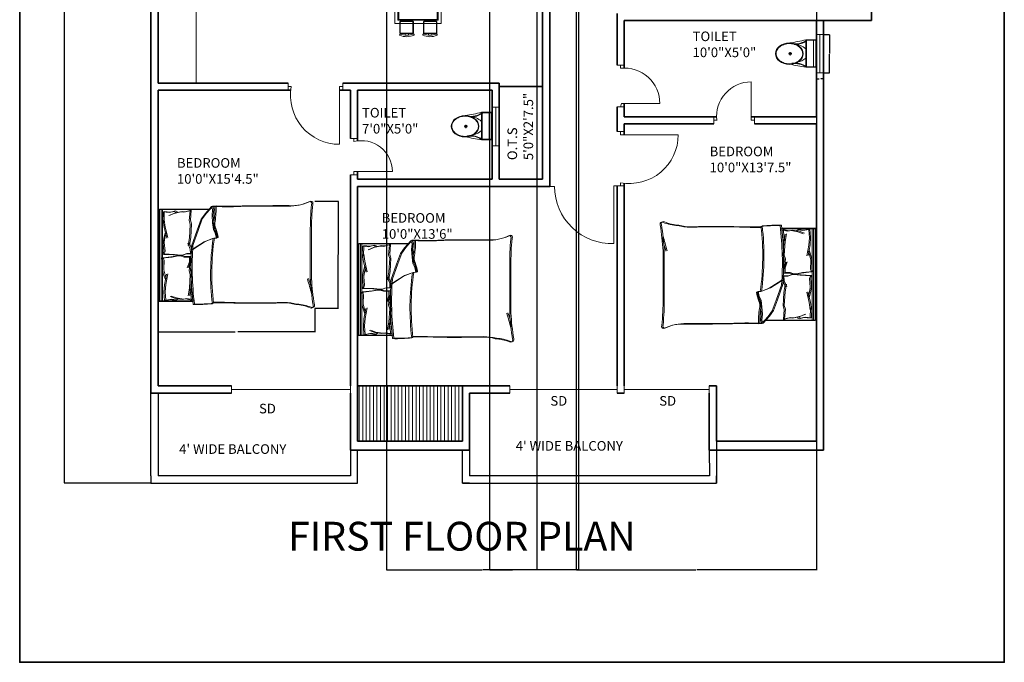
# Model space of a CAD drawing. Units: inches. Extents: x 1088 to 1703, y 668 to 1875.
# Tile 1 of 45: x 1088 to 1703, y 668 to 1069. Entities that reach past the tile are written whole.
import ezdxf

# ---------------------------------------------------------------- set-up
doc = ezdxf.new("R2010")
doc.units = ezdxf.units.IN
for name, color, linetype, lineweight in [('A-ANNO-DIMS', 2, 'Continuous', 18), ('A-ANNO-TEXT', 7, 'Continuous', 18), ('A-ANNO-TTLB', 7, 'Continuous', 35), ('A-AREA-IDEN', 7, 'Continuous', 18), ('A-DOOR', 4, 'Continuous', 18), ('A-FLOR-CASE', 8, 'Continuous', 18), ('A-FLOR-FIXT', 8, 'Continuous', 18), ('A-FLOR-HRAL', 7, 'Continuous', 25), ('A-FLOR-PATT', 252, 'Continuous', 13), ('A-FURN', 8, 'Continuous', 13), ('A-GLAZ', 4, 'Continuous', 18), ('A-WALL', 7, 'Continuous', 35)]:
    doc.layers.add(name, color=color, linetype=linetype, lineweight=lineweight)
doc.styles.get("Standard").update_dxf_attribs({"font": 'arial.ttf'})
doc.dimstyles.get("Standard").update_dxf_attribs({"dimtxt": 0.18, "dimasz": 0.18, "dimexe": 0.18, "dimexo": 0.0625, "dimgap": 0.09, "dimtad": 0, "dimtih": 1, "dimtoh": 1, "dimdec": 4, "dimzin": 0, "dimdsep": 46, "dimtxsty": 'Standard', "dimcen": 0.09, "dimadec": 0, "dimazin": 0, "dimtfac": 1, "dimtdec": 4, "dimtofl": 0, "dimtmove": 0, "dimatfit": 3, "dimfxl": 1, "dimtolj": 1, "dimtzin": 0, "dimarcsym": 0})

# ---------------------------------------------------------------- blocks, each defined once
blk = doc.blocks.new('A$C31115884')
for p, q in [((283, 498), (223, 498)), ((258, 466), (258, 523)), ((0, 200), (0, 0)), ((520, 200), (0, 200)), ((10, 190), (10, 10)), ((510, 190), (10, 190)), ((510, 10), (510, 190)), ((520, 0), (520, 200)), ((510, 54), (0, 54)), ((10, 10), (510, 10)), ((0, 0), (520, 0))]:
    blk.add_line(p, q)
blk.add_circle((256, 496), 23.6)
for centre, radius, start, end in [((2778, -205), 2807, 165.4549, 171.7133), ((-295, 403), 365, 324.2091, 9.3499), ((-295, 403), 375, 324.2091, 9.3499), ((139, 406), 293, 315.8436, 2.6563), ((806, 403), 375, 179.2036, 215.7909), ((806, 403), 365, 170.6501, 215.7909), ((3237, 905), 2807, 188.2867, 194.5451), ((384, 406), 293, 190.2774, 224.1564)]:
    blk.add_arc(centre, radius, start, end)
blk.add_ellipse((256, 510), major_axis=(0, -261), ratio=0.772727)
blk.add_open_spline([(256, 259), (263, 259), (270, 260), (288, 262), (299, 265), (320, 273), (330, 278), (350, 291), (360, 299), (378, 316), (386, 326), (402, 347), (409, 358), (421, 383), (427, 395), (436, 422), (440, 436), (445, 465), (447, 480), (448, 509), (448, 524), (445, 553), (443, 568), (436, 596), (432, 610), (422, 636), (416, 649), (402, 672), (395, 683), (379, 703), (370, 712), (351, 728), (341, 735), (321, 746), (310, 751), (289, 757), (278, 759), (256, 761), (245, 761), (223, 757), (212, 754), (191, 746), (181, 741), (161, 728), (151, 720), (133, 703), (125, 693), (110, 672), (103, 660), (90, 636), (85, 623), (76, 596), (72, 582), (67, 553), (66, 538), (64, 509), (65, 494), (68, 465), (70, 450), (77, 422), (81, 408), (91, 382), (97, 370), (111, 346), (118, 335), (135, 316), (144, 307), (162, 291), (172, 284), (193, 273), (203, 269), (225, 262), (236, 260), (250, 259), (253, 259), (256, 259)], degree=3, knots=[0, 0, 0, 0, 0.110105, 0.110105, 0.285049, 0.285049, 0.459994, 0.459994, 0.634938, 0.634938, 0.809882, 0.809882, 0.984827, 0.984827, 1.159771, 1.159771, 1.334715, 1.334715, 1.50966, 1.50966, 1.684604, 1.684604, 1.859549, 1.859549, 2.034493, 2.034493, 2.209437, 2.209437, 2.384382, 2.384382, 2.559326, 2.559326, 2.73427, 2.73427, 2.909215, 2.909215, 3.084159, 3.084159, 3.259103, 3.259103, 3.434048, 3.434048, 3.608992, 3.608992, 3.783936, 3.783936, 3.958881, 3.958881, 4.133825, 4.133825, 4.30877, 4.30877, 4.483714, 4.483714, 4.658658, 4.658658, 4.833603, 4.833603, 5.008547, 5.008547, 5.183491, 5.183491, 5.358436, 5.358436, 5.53338, 5.53338, 5.708324, 5.708324, 5.883269, 5.883269, 6.058213, 6.058213, 6.233158, 6.233158, 6.283185, 6.283185, 6.283185, 6.283185])
blk = doc.blocks.new('BED-DOUBLE')
for p, q in [((0.77, 61.73), (32.67, 61.73)), ((0.77, 4.44), (0.77, 61.73)), ((2.6, 4.44), (2.6, 61.73)), ((33.26, 63.38), (29.37, 58.94)), ((34.03, 63.65), (30.13, 59.21)), ((35.35, 63.48), (33.26, 63.38, 4.64)), ((34.01, 61.54), (33.26, 63.38)), ((33.63, 57.82), (34.01, 61.54)), ((36.12, 63.75), (34.03, 63.65, 4.64)), ((34.77, 61.81), (34.03, 63.65)), ((34.4, 58.1), (34.77, 61.81)), ((0, 61.46), (31.9, 61.46)), ((0, 4.17), (0, 61.46)), ((1.84, 4.17), (1.84, 61.46)), ((3.07, 60.08), (2.95, 53.6)), ((3.07, 60.08), (6.91, 59.62)), ((3.83, 60.35), (3.72, 53.87)), ((3.83, 60.35), (7.68, 59.9)), ((9.9, 59.12), (6.69, 57.7)), ((6.91, 59.62), (10, 60.34)), ((10.67, 59.39), (7.45, 57.97)), ((7.68, 59.9), (10.76, 60.61)), ((14.18, 60.08), (9.9, 59.12)), ((10, 60.34), (11.25, 59.72)), ((14.95, 60.35), (10.67, 59.39)), ((10.76, 60.61), (12.02, 59.99)), ((16.11, 59.85), (14.18, 60.08)), ((16.87, 60.12), (14.95, 60.35)), ((19.87, 60.78), (16.11, 59.85)), ((20.63, 61.05), (16.87, 60.12)), ((19.38, 54.63), (19.87, 60.78)), ((20.15, 54.9), (20.63, 61.05)), ((26.77, 55.41), (24.36, 48.73)), ((27.54, 55.68), (25.12, 49)), ((29.37, 58.94), (26.77, 55.41)), ((30.13, 59.21), (27.54, 55.68)), ((34.01, 53.18), (33.63, 57.82)), ((34.77, 53.46), (34.4, 58.1)), ((2.95, 53.6), (3.05, 54.8)), ((3.05, 54.8), (3.68, 50.25)), ((3.68, 50.25), (5.3, 43.75)), ((3.72, 53.87), (3.81, 55.08)), ((3.81, 55.08), (4.45, 50.52)), ((4.45, 50.52), (6.07, 44.03)), ((20.05, 52.28), (19.38, 54.63)), ((19.54, 43.87), (20.05, 52.28)), ((20.82, 52.55), (20.15, 54.9)), ((20.3, 44.15), (20.82, 52.55)), ((34.56, 49.1), (34.01, 53.18)), ((35.33, 49.37), (34.77, 53.46)), ((36.44, 46.96), (35.33, 49.37)), ((3.69, 44.52), (3.04, 41.01)), ((4.4, 47), (3.69, 44.52)), ((4.46, 44.79), (3.81, 41.28)), ((5.17, 47.27), (4.46, 44.79)), ((18.74, 39.04), (19.54, 43.87)), ((19.5, 39.31), (20.3, 44.15)), ((24.36, 48.73), (20.84, 38.73)), ((25.12, 49), (21.61, 39)), ((28.62, 41.3), (34.01, 43.34)), ((29.39, 41.57), (34.77, 43.62)), ((34.01, 43.34), (36.42, 43.71)), ((35.68, 46.68), (34.56, 49.1)), ((34.77, 43.62), (37.18, 43.99)), ((36.42, 43.71), (35.68, 46.68)), ((37.18, 43.99), (36.44, 46.96)), ((95, 18.06), (95, 47.57)), ((95.77, 18.33), (95.77, 47.84)), ((3.04, 41.01), (3.07, 40.62)), ((3.07, 40.62), (3.57, 35.31)), ((3.81, 41.28), (3.83, 40.9)), ((3.83, 40.9), (4.34, 35.59)), ((20.07, 36.87), (18.53, 40.55)), ((20.83, 37.14), (19.29, 40.82)), ((21.02, 34.2), (20.83, 37.14)), ((20.84, 36.28), (28.62, 41.3)), ((21.61, 36.55), (29.39, 41.57)), ((2.24, 31.15), (8.66, 31.84)), ((2.94, 29.42), (2.24, 31.15)), ((3.57, 35.31), (2.99, 33.54)), ((2.99, 33.54), (9.43, 33.25)), ((3.01, 31.42), (9.42, 32.12)), ((3.7, 29.69), (3.01, 31.42)), ((4.34, 35.59), (3.75, 33.81)), ((3.75, 33.81), (10.2, 33.52)), ((8.66, 31.84), (12.47, 32.54)), ((9.42, 32.12), (13.24, 32.81)), ((9.43, 33.25), (13.28, 32.79)), ((10.2, 33.52), (14.05, 33.07)), ((12.47, 32.54), (14.03, 32.54)), ((13.24, 32.81), (14.8, 32.81)), ((13.28, 32.79), (14.84, 32.89)), ((14.03, 32.54), (16.28, 31.84)), ((14.05, 33.07), (15.6, 33.17)), ((14.8, 32.81), (17.05, 32.12)), ((14.84, 32.89), (17.04, 33.72)), ((15.6, 33.17), (17.81, 34)), ((16.28, 31.84), (19.5, 31.84)), ((17.04, 33.72), (20.25, 33.93)), ((17.05, 32.12), (20.26, 32.12)), ((17.81, 34), (21.02, 34.2)), ((19.5, 31.84), (19.5, 28.9)), ((20.25, 33.93), (20.07, 36.87)), ((20.26, 32.12), (20.26, 29.17)), ((2.76, 24.09), (2.94, 29.42)), ((3.53, 24.36), (3.7, 29.69)), ((19.5, 28.9), (18.19, 25.13)), ((20.26, 29.17), (18.96, 25.4)), ((19.38, 23.24), (19.87, 29.39)), ((20.15, 23.51), (20.63, 29.67)), ((2.76, 23.7), (2.76, 24.09)), ((3.63, 20.24), (2.76, 23.7)), ((3.53, 23.98), (3.53, 24.36)), ((4.4, 20.51), (3.53, 23.98)), ((4.5, 17.81), (3.63, 20.24)), ((3.98, 14.52), (5.19, 21.1)), ((5.26, 18.08), (4.4, 20.51)), ((4.74, 14.79), (5.96, 21.38)), ((20.05, 20.89), (19.38, 23.24)), ((19.54, 12.48), (20.05, 20.89)), ((20.82, 21.16), (20.15, 23.51)), ((20.3, 12.76), (20.82, 21.16)), ((3.63, 9.93), (3.98, 14.52)), ((4.4, 10.21), (4.74, 14.79)), ((18.74, 7.65), (19.54, 12.48)), ((19.5, 7.92), (20.3, 12.76)), ((19.54, 12.48), (19.92, 11.13)), ((20.3, 12.76), (20.69, 11.4)), ((3.61, 9.81), (3.63, 9.93)), ((4, 4.67), (3.61, 9.81)), ((4.37, 10.08), (4.4, 10.21)), ((4.77, 4.95), (4.37, 10.08)), ((10.74, 6.06), (7.44, 7.27)), ((11.5, 6.33), (8.21, 7.54)), ((15.84, 5.64), (11.5, 6.33)), ((19.92, 11.13), (20.79, 5.02)), ((20.69, 11.4), (21.56, 5.29)), ((21.71, 4.17), (0, 4.17)), ((22.48, 4.44), (0.77, 4.44)), ((3.98, 4.67), (7.79, 5.36)), ((4.74, 4.94), (8.56, 5.64)), ((7.79, 5.36), (10.91, 4.84)), ((8.56, 5.64), (11.68, 5.12)), ((15.07, 5.36), (10.74, 6.06)), ((10.91, 4.84), (12.12, 5.54)), ((11.68, 5.12), (12.89, 5.81)), ((16.98, 5.71), (15.07, 5.36)), ((17.74, 5.98), (15.84, 5.64)), ((20.79, 5.02), (16.98, 5.71)), ((21.56, 5.29), (17.74, 5.98))]:
    blk.add_line(p, q)
for centre, radius, start, end in [((-7.98, 61.53), 43.38, 349.87628, 2.56571), ((43.54, 218.51), 155.25, 266.97912, 273.83645), ((-7.21, 61.81), 43.38, 349.87628, 2.56571), ((44.3, 218.78), 155.25, 266.97912, 273.83645), ((81.31, -5405.34), 5469.02, 90.00217, 90.28689), ((82.07, -5405.07), 5469.02, 90.00217, 90.28689), ((82.32, 91.3), 27.65, 267.47136, 296.46809), ((83.09, 91.58), 27.65, 267.47136, 296.46809), ((94.55, 65.23), 1.32, 332.65876, 86.02002), ((254.49, 49.34), 159.5, 174.4998, 180.63509), ((95.32, 65.5), 1.32, 332.65876, 86.02002), ((255.26, 49.61), 159.5, 174.4998, 180.63509), ((42.04, 52.44), 7.46, 168.6608, 203.73842), ((1.78, 37.35), 35.55, 10.66171, 19.88058), ((42.81, 52.72), 7.46, 168.6608, 203.73842), ((2.54, 37.62), 35.55, 10.66171, 19.88058), ((187.4, 21.29), 154.68, 171.78449, 186.90062), ((188.17, 21.56), 154.68, 171.78449, 186.90062), ((36.49, 43.92), 0.221, 250.24637, 1.13765), ((37.26, 44.2), 0.221, 250.24637, 1.13765), ((218.25, 25.61), 197.77, 176.08655, 186.78213), ((219.02, 25.88), 197.77, 176.08655, 186.78213), ((-28.43, -20.65), 127.63, 13.38322, 17.70533), ((-27.66, -20.37), 127.63, 13.38322, 17.70533), ((240.78, 25.69), 145.97, 182.99578, 189.40907), ((241.54, 25.96), 145.97, 182.99578, 189.40907), ((24.09, 102.1), 99.87, 268.72178, 275.60397), ((24.86, 102.37), 99.87, 268.72178, 275.60397), ((37.37, -200.58), 203.94, 88.4762, 91.00819), ((38.14, -200.3), 203.94, 88.4762, 91.00819), ((60.68, 581.23), 578.22, 268.22771, 271.71854), ((61.45, 581.51), 578.22, 268.22771, 271.71854), ((77.34, -32.25), 35.53, 76.06484, 88.91125), ((78.11, -31.97), 35.53, 76.06484, 88.91125), ((84.25, -25.97), 28.25, 67.97508, 86.652), ((85.02, -25.69), 28.25, 67.97508, 86.652), ((95.57, 1.3), 1.31, 236.17358, 23.47814), ((96.34, 1.58), 1.31, 236.17358, 23.47814)]:
    blk.add_arc(centre, radius, start, end)
blk = doc.blocks.new('TABLE-DINING-RECT')
for points in [[(0, 17.41), (29.01, 17.41), (29.01, 0), (0, 0)], [(1.93, 15.47), (27.08, 15.47), (27.08, 1.93), (1.93, 1.93)], [(2.51, 14.89), (26.5, 14.89), (26.5, 2.51), (2.51, 2.51)]]:
    blk.add_lwpolyline(points, close=True)
blk = doc.blocks.new('CHAIR-DINING')
for points in [[(7.77, 8.29, 0.414214), (7.26, 8.81), (0.51, 8.81, 0.414214), (0, 8.29), (0, 0.96, 0.414214), (0.51, 0.44), (7.26, 0.44, 0.414214), (7.77, 0.96), (7.77, 8.29)], [(8.09, 8.52, -0.175809), (8.03, 0.62, 0.578392), (8.69, 0.02, 0.214524), (8.81, 8.94, 0.552014), (8.09, 8.52, -0.065079)], [(7.77, 3.53), (8.7, 3.53, -0.064759)]]:
    blk.add_lwpolyline(points, format="xyb")
blk.add_lwpolyline([(7.54, 8.29), (7.54, 1.19, -0.414214), (7.03, 0.68), (0.74, 0.68, -0.414214), (0.23, 1.19), (0.23, 8.29, -0.512069), (0.74, 8.58), (7.03, 8.58, -0.512069)], format="xyb", close=True)
blk.add_lwpolyline([(8.72, 5.59), (7.77, 5.59)])
blk = doc.blocks.new('WIN-24-RETURN')
for p, q in [((0, 24), (4.5, 24)), ((4.5, 24), (2.25, 24)), ((2.25, 24), (2.25, 0)), ((4.5, 0), (0, 0)), ((2.25, 0), (4.5, 0))]:
    blk.add_line(p, q)
blk = doc.blocks.new('*D10')
at = {"layer": 'A-ANNO-DIMS', "color": 0, "lineweight": -2, "transparency": 16777216}
for p, q in [((1174.84, 888.9), (1174.84, 874.12)), ((1272.61, 888.9), (1272.61, 874.12)), ((1175.02, 874.3), (1222.91, 874.3)), ((1272.43, 874.3), (1224.54, 874.3))]:
    blk.add_line(p, q, dxfattribs=at)
at = {"layer": 'A-ANNO-DIMS', "color": 0, "transparency": 16777216}
for points in [[(1175.02, 874.33), (1175.02, 874.27), (1174.84, 874.3)], [(1272.43, 874.33), (1272.43, 874.27), (1272.61, 874.3)]]:
    blk.add_solid(points, dxfattribs=at)
at = {"layer": 'Defpoints', "color": 0, "transparency": 16777216}
for p in [(1174.84, 888.97), (1272.61, 888.97), (1272.61, 874.3)]:
    blk.add_point(p, dxfattribs=at)
at = {"layer": 'A-ANNO-DIMS', "color": 0, "transparency": 16777216, "insert": (1223.73, 874.3), "char_height": 0.18, "attachment_point": 5}
blk.add_mtext('\\A1;BED 98 TYP.', dxfattribs=at)
blk = doc.blocks.new('*D11')
at = {"layer": 'A-ANNO-DIMS', "color": 0, "lineweight": -2, "transparency": 16777216}
for p, q in [((1272.67, 955.89), (1287.45, 955.89)), ((1287.27, 955.71), (1287.27, 922.61)), ((1287.27, 889.15), (1287.27, 922.25)), ((1272.67, 888.97), (1287.45, 888.97))]:
    blk.add_line(p, q, dxfattribs=at)
at = {"layer": 'A-ANNO-DIMS', "color": 0, "transparency": 16777216}
for points in [[(1287.24, 955.71), (1287.3, 955.71), (1287.27, 955.89)], [(1287.24, 889.15), (1287.3, 889.15), (1287.27, 888.97)]]:
    blk.add_solid(points, dxfattribs=at)
at = {"layer": 'Defpoints', "color": 0, "transparency": 16777216}
for p in [(1272.61, 955.89), (1287.27, 955.89), (1272.61, 888.97)]:
    blk.add_point(p, dxfattribs=at)
at = {"layer": 'A-ANNO-DIMS', "color": 0, "transparency": 16777216, "insert": (1287.27, 922.43), "char_height": 0.18, "attachment_point": 5}
blk.add_mtext('\\A1;67 TYP.', dxfattribs=at)
blk = doc.blocks.new('*D18')
at = {"layer": 'A-ANNO-DIMS', "color": 0, "lineweight": -2, "transparency": 16777216}
for p, q in [((1590.41, 1059.85), (1594.12, 1059.85)), ((1593.94, 1059.67), (1593.94, 1048.03)), ((1593.94, 1036.03), (1593.94, 1047.66)), ((1590.41, 1035.85), (1594.12, 1035.85))]:
    blk.add_line(p, q, dxfattribs=at)
at = {"layer": 'A-ANNO-DIMS', "color": 0, "transparency": 16777216}
for points in [[(1593.91, 1059.67), (1593.97, 1059.67), (1593.94, 1059.85)], [(1593.91, 1036.03), (1593.97, 1036.03), (1593.94, 1035.85)]]:
    blk.add_solid(points, dxfattribs=at)
at = {"layer": 'Defpoints', "color": 0, "transparency": 16777216}
for p in [(1590.34, 1059.85), (1593.94, 1059.85), (1590.34, 1035.85)]:
    blk.add_point(p, dxfattribs=at)
at = {"layer": 'A-ANNO-DIMS', "color": 0, "transparency": 16777216, "insert": (1593.94, 1047.85), "char_height": 0.18, "attachment_point": 5}
blk.add_mtext('\\A1;WINDOW 24 TYP.', dxfattribs=at)
blk = doc.blocks.new('*D19')
at = {"layer": 'A-ANNO-DIMS', "color": 0, "lineweight": -2, "transparency": 16777216}
for p, q in [((1585.84, 1035.78), (1585.84, 1032.07)), ((1590.34, 1035.78), (1590.34, 1032.07)), ((1586.02, 1032.25), (1587.64, 1032.25)), ((1590.16, 1032.25), (1588.55, 1032.25))]:
    blk.add_line(p, q, dxfattribs=at)
at = {"layer": 'A-ANNO-DIMS', "color": 0, "transparency": 16777216}
for points in [[(1586.02, 1032.28), (1586.02, 1032.22), (1585.84, 1032.25)], [(1590.16, 1032.28), (1590.16, 1032.22), (1590.34, 1032.25)]]:
    blk.add_solid(points, dxfattribs=at)
at = {"layer": 'Defpoints', "color": 0, "transparency": 16777216}
for p in [(1585.84, 1035.85), (1590.34, 1035.85), (1590.34, 1032.25)]:
    blk.add_point(p, dxfattribs=at)
at = {"layer": 'A-ANNO-DIMS', "color": 0, "transparency": 16777216, "insert": (1588.09, 1032.25), "char_height": 0.18, "attachment_point": 5}
blk.add_mtext('\\A1;5 TYP.', dxfattribs=at)
blk = doc.blocks.new('*D29')
at = {"layer": 'A-ANNO-DIMS', "color": 0, "lineweight": -2, "transparency": 16777216}
for p, q in [((1170.28, 1803.56), (1116.11, 1803.56)), ((1116.29, 1803.38), (1116.29, 1291.85)), ((1116.29, 779.96), (1116.29, 1291.49)), ((1170.28, 779.78), (1116.11, 779.78))]:
    blk.add_line(p, q, dxfattribs=at)
at = {"layer": 'A-ANNO-DIMS', "color": 0, "transparency": 16777216}
for points in [[(1116.26, 1803.38), (1116.32, 1803.38), (1116.29, 1803.56)], [(1116.26, 779.96), (1116.32, 779.96), (1116.29, 779.78)]]:
    blk.add_solid(points, dxfattribs=at)
at = {"layer": 'Defpoints', "color": 0, "transparency": 16777216}
for p in [(1116.29, 1803.56), (1170.34, 1803.56), (1170.34, 779.78)]:
    blk.add_point(p, dxfattribs=at)
at = {"layer": 'A-ANNO-DIMS', "color": 0, "transparency": 16777216, "insert": (1116.29, 1291.67), "char_height": 0.18, "attachment_point": 5}
blk.add_mtext('\\A1;1023.8', dxfattribs=at)
blk = doc.blocks.new('*D31')
at = {"layer": 'A-ANNO-DIMS', "color": 0, "lineweight": -2, "transparency": 16777216}
for p, q in [((1435.84, 1326.5), (1435.84, 725.55)), ((1585.84, 1326.5), (1585.84, 725.55)), ((1436.02, 725.73), (1510.56, 725.73)), ((1585.66, 725.73), (1511.12, 725.73))]:
    blk.add_line(p, q, dxfattribs=at)
at = {"layer": 'A-ANNO-DIMS', "color": 0, "transparency": 16777216}
for points in [[(1436.02, 725.76), (1436.02, 725.7), (1435.84, 725.73)], [(1585.66, 725.76), (1585.66, 725.7), (1585.84, 725.73)]]:
    blk.add_solid(points, dxfattribs=at)
at = {"layer": 'Defpoints', "color": 0, "transparency": 16777216}
for p in [(1435.84, 1326.56), (1585.84, 1326.56), (1585.84, 725.73)]:
    blk.add_point(p, dxfattribs=at)
at = {"layer": 'A-ANNO-DIMS', "color": 0, "transparency": 16777216, "insert": (1510.84, 725.73), "char_height": 0.18, "attachment_point": 5}
blk.add_mtext('\\A1;150', dxfattribs=at)
blk = doc.blocks.new('*D37')
at = {"layer": 'A-ANNO-DIMS', "color": 0, "lineweight": -2, "transparency": 16777216}
for p, q in [((1381.79, 1151.2), (1381.79, 725.55)), ((1411.2, 1151.2), (1411.2, 725.55)), ((1381.97, 725.73), (1396.11, 725.73)), ((1411.02, 725.73), (1396.87, 725.73))]:
    blk.add_line(p, q, dxfattribs=at)
at = {"layer": 'A-ANNO-DIMS', "color": 0, "transparency": 16777216}
for points in [[(1381.97, 725.76), (1381.97, 725.7), (1381.79, 725.73)], [(1411.02, 725.76), (1411.02, 725.7), (1411.2, 725.73)]]:
    blk.add_solid(points, dxfattribs=at)
at = {"layer": 'Defpoints', "color": 0, "transparency": 16777216}
for p in [(1381.79, 1151.26), (1411.2, 1151.26), (1411.2, 725.73)]:
    blk.add_point(p, dxfattribs=at)
at = {"layer": 'A-ANNO-DIMS', "color": 0, "transparency": 16777216, "insert": (1396.49, 725.73), "char_height": 0.18, "attachment_point": 5}
blk.add_mtext('\\A1;29.41', dxfattribs=at)
blk = doc.blocks.new('*D38')
at = {"layer": 'A-ANNO-DIMS', "color": 0, "lineweight": -2, "transparency": 16777216}
for p, q in [((1317.34, 1736.94), (1317.34, 725.55)), ((1437.34, 1736.94), (1437.34, 725.55)), ((1317.52, 725.73), (1377.06, 725.73)), ((1437.16, 725.73), (1377.62, 725.73))]:
    blk.add_line(p, q, dxfattribs=at)
at = {"layer": 'A-ANNO-DIMS', "color": 0, "transparency": 16777216}
for points in [[(1317.52, 725.76), (1317.52, 725.7), (1317.34, 725.73)], [(1437.16, 725.76), (1437.16, 725.7), (1437.34, 725.73)]]:
    blk.add_solid(points, dxfattribs=at)
at = {"layer": 'Defpoints', "color": 0, "transparency": 16777216}
for p in [(1317.34, 1737.01), (1437.34, 1737.01), (1437.34, 725.73)]:
    blk.add_point(p, dxfattribs=at)
at = {"layer": 'A-ANNO-DIMS', "color": 0, "transparency": 16777216, "insert": (1377.34, 725.73), "char_height": 0.18, "attachment_point": 5}
blk.add_mtext('\\A1;120', dxfattribs=at)

msp = doc.modelspace()

# ---------------------------------------------------------------- hatches: boundary and pattern name
at = {"layer": 'A-FLOR-PATT'}
h = msp.add_hatch(dxfattribs=at)
h.set_pattern_fill('ANSI31', color=256, scale=0.700077, angle=45, style=0)
h.paths.add_polyline_path([(1299.345, 806.058), (1364.804, 806.058), (1364.804, 840.558), (1299.345, 840.558)])

# ---------------------------------------------------------------- linework, layer by layer
at = {"layer": 'A-ANNO-TTLB'}
msp.add_lwpolyline([(1088.369, 1874.677), (1703.181, 1874.677), (1703.181, 667.947), (1088.369, 667.947)], close=True, dxfattribs=at)
at = {"layer": 'A-DOOR'}
for p, q in [((1461.345, 1040.808), (1465.845, 1040.808)), ((1465.845, 1040.808), (1461.345, 1040.808)), ((1461.345, 1040.808), (1463.595, 1040.808)), ((1463.595, 1040.808), (1463.595, 1038.808)), ((1255.914, 1025.058), (1255.914, 1029.558)), ((1255.914, 1029.558), (1255.914, 1027.308)), ((1255.914, 1027.308), (1257.914, 1027.308)), ((1290.103, 1027.308), (1288.103, 1027.308)), ((1288.103, 1027.308), (1288.103, 991.308)), ((1290.103, 1025.058), (1290.103, 1029.558)), ((1290.103, 1029.558), (1290.103, 1027.308)), ((1545.172, 1006.308), (1545.172, 1030.308)), ((1461.345, 1014.775), (1465.845, 1014.775)), ((1463.595, 1014.775), (1464.095, 1016.711)), ((1465.845, 1014.775), (1463.595, 1014.775)), ((1464.095, 1016.711), (1488.095, 1016.711)), ((1521.883, 1008.558), (1521.883, 1004.058)), ((1547.172, 1008.558), (1547.172, 1004.058)), ((1521.883, 1004.058), (1521.883, 1006.308)), ((1521.883, 1006.308), (1523.883, 1006.308)), ((1547.172, 1006.308), (1545.172, 1006.308)), ((1547.172, 1004.058), (1547.172, 1006.308)), ((1465.845, 999.326), (1461.345, 999.326)), ((1461.345, 999.326), (1463.595, 999.326)), ((1463.595, 999.326), (1463.595, 997.326)), ((1463.595, 997.326), (1499.595, 997.326)), ((1294.845, 994.994), (1299.345, 994.994)), ((1299.345, 994.994), (1297.095, 994.994)), ((1297.095, 994.994), (1297.095, 992.994)), ((1299.345, 972.333), (1294.845, 972.333)), ((1294.845, 972.333), (1297.095, 972.333)), ((1297.095, 972.333), (1297.095, 974.333)), ((1297.095, 974.333), (1321.095, 974.333)), ((1461.345, 965.344), (1459.345, 965.344)), ((1459.345, 965.344), (1459.345, 929.344)), ((1465.845, 965.344), (1461.345, 965.344)), ((1461.345, 965.344), (1463.595, 965.344)), ((1463.595, 965.344), (1463.595, 967.344)), ((1419.345, 965.058), (1422.345, 965.058)), ((1220.612, 840.558), (1220.612, 836.058)), ((1220.612, 838.308), (1294.845, 838.308)), ((1294.845, 840.558), (1294.845, 836.058)), ((1394.503, 836.058), (1394.503, 840.558)), ((1394.503, 838.308), (1461.345, 838.308)), ((1461.345, 840.558), (1461.345, 836.058)), ((1465.845, 840.558), (1465.845, 836.058)), ((1465.845, 838.308), (1518.965, 838.308)), ((1518.965, 836.058), (1518.965, 840.558))]:
    msp.add_line(p, q, dxfattribs=at)
for centre, radius, start, end in [((1465.88, 1016.711), 22.215, 0, 95.905414), ((1288.103, 1021.966), 30.658, 169.965011, 270), ((1545.172, 1008.609), 21.699, 90, 186.087007), ((1469.11, 997.326), 30.485, 259.577932, 360), ((1301.84, 974.333), 19.255, 0, 104.267411), ((1458.082, 965.058), 35.737, 180, 272.025225)]:
    msp.add_arc(centre, radius, start, end, dxfattribs=at)
at = {"layer": 'A-FLOR-CASE'}
msp.add_line((1198.631, 1029.558), (1198.631, 1167.334), dxfattribs=at)
at = {"layer": 'A-FLOR-HRAL'}
for p, q in [((1170.345, 784.279), (1170.345, 836.058)), ((1170.345, 836.058), (1174.845, 836.058)), ((1174.845, 836.058), (1174.845, 784.279)), ((1523.465, 806.058), (1523.465, 779.779)), ((1294.845, 800.472), (1294.845, 784.279)), ((1299.345, 779.779), (1299.345, 800.472)), ((1364.804, 779.779), (1364.804, 800.472)), ((1369.304, 800.472), (1369.304, 784.279)), ((1518.965, 800.472), (1519.128, 784.279)), ((1518.965, 800.472), (1523.465, 800.472)), ((1170.345, 784.279), (1170.345, 779.779)), ((1294.845, 784.279), (1174.845, 784.279)), ((1519.128, 784.279), (1369.304, 784.279)), ((1523.465, 779.779), (1523.465, 784.279)), ((1170.345, 779.779), (1294.845, 779.779)), ((1294.845, 779.779), (1299.345, 779.779)), ((1364.804, 779.779), (1523.465, 779.779)), ((1369.304, 779.779), (1364.804, 779.779)), ((1369.304, 779.779), (1519.173, 779.779))]:
    msp.add_line(p, q, dxfattribs=at)
at = {"layer": 'A-FURN'}
for points in [[(1348.323, 1060.419, 0.4142136), (1348.836, 1060.932), (1348.836, 1067.677, 0.4142136), (1348.323, 1068.19), (1340.987, 1068.19, 0.4142136), (1340.474, 1067.677), (1340.474, 1060.932, 0.4142136), (1340.987, 1060.419), (1348.323, 1060.419)], [(1348.554, 1060.101, -0.1758093), (1340.652, 1060.161, 0.5783921), (1340.053, 1059.503, 0.2145244), (1348.973, 1059.383, 0.552014), (1348.554, 1060.101, -0.065079)], [(1343.564, 1060.419), (1343.564, 1059.491, -0.0647586)]]:
    msp.add_lwpolyline(points, format="xyb", dxfattribs=at)
msp.add_lwpolyline([(1348.32, 1060.65), (1341.218, 1060.65, -0.4142136), (1340.705, 1061.163), (1340.705, 1067.446, -0.4142136), (1341.218, 1067.959), (1348.32, 1067.959, -0.5120695), (1348.605, 1067.446), (1348.605, 1061.163, -0.5120695)], format="xyb", close=True, dxfattribs=at)
msp.add_lwpolyline([(1345.617, 1059.474), (1345.617, 1060.419)], dxfattribs=at)
at = {"layer": 'A-WALL'}
for p, q in [((1170.345, 1803.558), (1170.345, 836.058)), ((1414.845, 1291.827), (1414.845, 1027.308)), ((1419.345, 965.058), (1419.345, 1291.827)), ((1174.845, 1189.644), (1174.845, 1029.558)), ((1620.345, 1185.558), (1620.345, 1068.558)), ((1414.845, 1154.058), (1414.845, 969.558)), ((1419.345, 965.058), (1419.345, 1154.058)), ((1461.345, 1073.058), (1461.345, 1040.808)), ((1174.845, 1065.144), (1174.845, 1029.558)), ((1465.845, 1068.558), (1585.845, 1068.558)), ((1465.845, 1038.926), (1465.845, 1068.558)), ((1620.345, 1068.558), (1548.345, 1068.558)), ((1585.845, 1068.558), (1585.845, 1008.558)), ((1585.845, 1068.558), (1585.845, 1008.558)), ((1590.345, 1068.558), (1590.345, 836.058)), ((1174.845, 1029.558), (1255.914, 1029.558)), ((1290.103, 1029.558), (1294.845, 1029.558)), ((1294.845, 1029.558), (1299.345, 1029.558)), ((1299.345, 1029.558), (1383.345, 1029.558)), ((1387.845, 1029.558), (1383.345, 1029.558)), ((1383.345, 1029.558), (1387.845, 1029.558)), ((1387.845, 969.558), (1387.845, 1029.558)), ((1387.845, 1029.558), (1387.845, 1025.058)), ((1387.845, 1027.308), (1414.845, 1027.308)), ((1257.601, 1025.058), (1174.845, 1025.058)), ((1174.845, 1025.058), (1174.845, 840.558)), ((1174.845, 1025.058), (1174.845, 840.558)), ((1294.845, 1025.058), (1288.103, 1025.058)), ((1294.845, 994.994), (1294.845, 1025.058)), ((1299.345, 1025.058), (1299.345, 993.425)), ((1383.345, 1025.058), (1299.345, 1025.058)), ((1383.345, 1025.058), (1383.345, 969.558)), ((1461.345, 1014.775), (1461.345, 1008.558)), ((1465.845, 1008.558), (1465.845, 1016.711)), ((1461.345, 1008.558), (1461.345, 1004.058)), ((1523.473, 1008.558), (1465.845, 1008.558)), ((1585.845, 1008.558), (1545.172, 1008.558)), ((1461.345, 1004.058), (1461.345, 999.326)), ((1465.845, 1004.058), (1521.883, 1004.058)), ((1465.845, 997.326), (1465.845, 1004.058)), ((1547.172, 1004.058), (1585.845, 1004.058)), ((1585.845, 1004.058), (1585.845, 836.058)), ((1585.845, 1004.058), (1585.845, 840.558)), ((1294.845, 840.558), (1294.845, 972.333)), ((1299.345, 974.333), (1299.345, 969.558)), ((1383.345, 969.558), (1299.345, 969.558)), ((1414.845, 969.558), (1387.845, 969.558)), ((1461.345, 965.344), (1461.345, 840.558)), ((1465.845, 840.558), (1465.845, 967.016)), ((1299.345, 965.058), (1383.345, 965.058)), ((1299.345, 965.058), (1299.345, 836.058)), ((1383.345, 965.058), (1387.845, 965.058)), ((1387.845, 965.058), (1419.345, 965.058)), ((1461.345, 876.144), (1461.345, 880.644)), ((1174.845, 840.558), (1220.612, 840.558)), ((1364.804, 840.558), (1299.345, 840.558)), ((1299.345, 840.558), (1300.345, 840.558)), ((1369.304, 840.558), (1364.804, 840.558)), ((1364.804, 840.558), (1364.804, 806.058)), ((1394.503, 840.558), (1369.304, 840.558)), ((1523.465, 840.558), (1518.965, 840.558)), ((1523.465, 806.058), (1523.465, 840.558)), ((1170.345, 836.058), (1220.612, 836.058)), ((1294.845, 836.058), (1294.845, 800.472)), ((1299.345, 836.058), (1299.345, 806.058)), ((1299.345, 836.058), (1299.345, 806.058)), ((1369.304, 800.472), (1369.304, 836.058)), ((1369.304, 836.058), (1394.503, 836.058)), ((1461.345, 836.058), (1465.845, 836.058)), ((1518.965, 836.058), (1518.965, 800.472)), ((1518.965, 836.058), (1518.965, 806.058)), ((1585.845, 836.058), (1585.845, 806.058)), ((1590.345, 800.472), (1590.345, 836.058)), ((1299.345, 806.058), (1364.804, 806.058)), ((1523.465, 806.058), (1585.845, 806.058)), ((1369.304, 800.472), (1294.845, 800.472)), ((1590.345, 800.472), (1518.965, 800.472))]:
    msp.add_line(p, q, dxfattribs=at)

# ---------------------------------------------------------------- block references
at = {"layer": 'A-FLOR-FIXT', "xscale": 0.0330640103915726, "yscale": 0.0330640103915726, "zscale": 0.0330640103915726, "rotation": 89.99999999999996}
for p in [(1585.845, 1039.383), (1383.345, 994.092)]:
    msp.add_blockref('A$C31115884', p, dxfattribs=at)
at = {"layer": 'A-FURN'}
for name, p in [('TABLE-DINING-RECT', (1322.51, 1066.8)), ('BED-DOUBLE', (1174.845, 889.07)), ('BED-DOUBLE', (1299.345, 867.745))]:
    msp.add_blockref(name, p, dxfattribs=at)
at = {"layer": 'A-FURN', "extrusion": (0, 0, -1), "zscale": -1, "rotation": 270.0000017090659}
msp.add_blockref('CHAIR-DINING', (-1334.622, 1068.19), dxfattribs=at)
at = {"layer": 'A-FURN', "rotation": 180}
msp.add_blockref('BED-DOUBLE', (1585.845, 943.054), dxfattribs=at)
at = {"layer": 'A-GLAZ'}
for p in [(1585.845, 1035.846), (1383.345, 990.415)]:
    msp.add_blockref('WIN-24-RETURN', p, dxfattribs=at)

# ---------------------------------------------------------------- texts
at = {"layer": 'A-ANNO-TEXT', "char_height": 6, "attachment_point": 1}
for s, width, insert in [('SD ', 27.4142, (1419.747, 834.155)), ('SD ', 27.4142, (1487.743, 834.155)), ('SD', 65.83698, (1237.813, 829.336))]:
    msp.add_mtext_dynamic_manual_height_columns(s, width=width, gutter_width=12.5, heights=[0], dxfattribs=dict(at, insert=insert))
at = {"layer": 'A-ANNO-TTLB', "insert": (1255.879, 755.65), "char_height": 18, "attachment_point": 1}
msp.add_mtext_dynamic_manual_height_columns('FIRST FLOOR PLAN', width=401.20715, gutter_width=12.5, heights=[0], dxfattribs=at)
at = {"layer": 'A-AREA-IDEN', "char_height": 6, "attachment_point": 1}
for s, width, insert in [('TOILET\\P10\'0"X5\'0"', 79.3055, (1508.561, 1061.717)), ('TOILET\\P7\'0"X5\'0"', 72.13056, (1302.143, 1014.04)), ('BEDROOM\\P10\'0"X13\'7.5"', 91.23234, (1519.191, 989.871)), ('BEDROOM\\P10\'0"X15\'4.5"', 121.13336, (1186.576, 982.695)), ('BEDROOM\\P10\'0"X13\'6"', 246.69188, (1314.442, 948.345)), ("4' WIDE BALCONY", 141.17895, (1398.119, 806.058)), ("4' WIDE BALCONY", 130.91994, (1187.968, 804.075))]:
    msp.add_mtext_dynamic_manual_height_columns(s, width=width, gutter_width=12.5, heights=[0], dxfattribs=dict(at, insert=insert))
at = {"layer": 'A-AREA-IDEN', "insert": (1392.968, 981.434), "char_height": 6, "attachment_point": 1, "rotation": 90}
msp.add_mtext_dynamic_manual_height_columns('O.T.S\\P5\'0"X2\'7.5"', width=65.99872, gutter_width=12.5, heights=[0], dxfattribs=at)

# ---------------------------------------------------------------- dimensions: what is measured, and where the dimension line sits
at = {"layer": 'A-ANNO-DIMS'}
dim = msp.add_linear_dim(base=(1116.295, 1803.558), p1=(1170.345, 779.779), p2=(1170.345, 1803.558), angle=90, dimstyle='Standard', override={"dimdec": 1, "dimlfac": 1, "dimrnd": 0, "dimzin": 0, "dimdsep": 46, "dimlunit": 2}, dxfattribs=at)
dim.commit()
dim.dimension.update_dxf_attribs({"geometry": '*D29', "text_midpoint": (1116.295, 1291.669)})
for base, p1, p2, override, picture, middle in [((1437.345, 725.729), (1317.345, 1737.007), (1437.345, 1737.007), {"dimdec": 0, "dimlfac": 1, "dimrnd": 0, "dimzin": 0, "dimdsep": 46, "dimlunit": 2}, '*D38', (1377.345, 725.729)), ((1585.845, 725.729), (1435.845, 1326.558), (1585.845, 1326.558), {"dimdec": 0, "dimlfac": 1, "dimrnd": 0, "dimzin": 0, "dimdsep": 46, "dimlunit": 2}, '*D31', (1510.845, 725.729)), ((1411.198, 725.729), (1381.786, 1151.259), (1411.198, 1151.259), {"dimdec": 2, "dimlfac": 1, "dimrnd": 0, "dimzin": 0, "dimdsep": 46, "dimlunit": 2}, '*D37', (1396.492, 725.729))]:
    dim = msp.add_linear_dim(base=base, p1=p1, p2=p2, dimstyle='Standard', override=override, dxfattribs=at)
    dim.commit()
    dim.dimension.update_dxf_attribs({"geometry": picture, "text_midpoint": middle})
for base, p1, p2, text, picture, middle in [((1593.945, 1059.846), (1590.345, 1035.846), (1590.345, 1059.846), 'WINDOW <> TYP.', '*D18', (1593.945, 1047.846)), ((1287.275, 955.893), (1272.61, 888.967), (1272.61, 955.893), '<> TYP.', '*D11', (1287.275, 922.43))]:
    dim = msp.add_linear_dim(base=base, p1=p1, p2=p2, angle=90, text=text, dimstyle='Standard', override={"dimdec": 0, "dimlfac": 1, "dimrnd": 0, "dimzin": 0, "dimdsep": 46, "dimlunit": 2}, dxfattribs=at)
    dim.commit()
    dim.dimension.update_dxf_attribs({"geometry": picture, "text_midpoint": middle})
for base, p1, p2, text, picture, middle in [((1590.344800082, 1032.246106164), (1585.844800082, 1035.846106164), (1590.344800082, 1035.846106164), '<> TYP.', '*D19', (1588.094800082, 1032.246106164)), ((1272.61, 874.303), (1174.845, 888.967), (1272.61, 888.967), 'BED <> TYP.', '*D10', (1223.727, 874.303))]:
    dim = msp.add_linear_dim(base=base, p1=p1, p2=p2, text=text, dimstyle='Standard', override={"dimdec": 0, "dimlfac": 1, "dimrnd": 0, "dimzin": 0, "dimdsep": 46, "dimlunit": 2}, dxfattribs=at)
    dim.commit()
    dim.dimension.update_dxf_attribs({"geometry": picture, "text_midpoint": middle})

doc.saveas('drawing.dxf')
